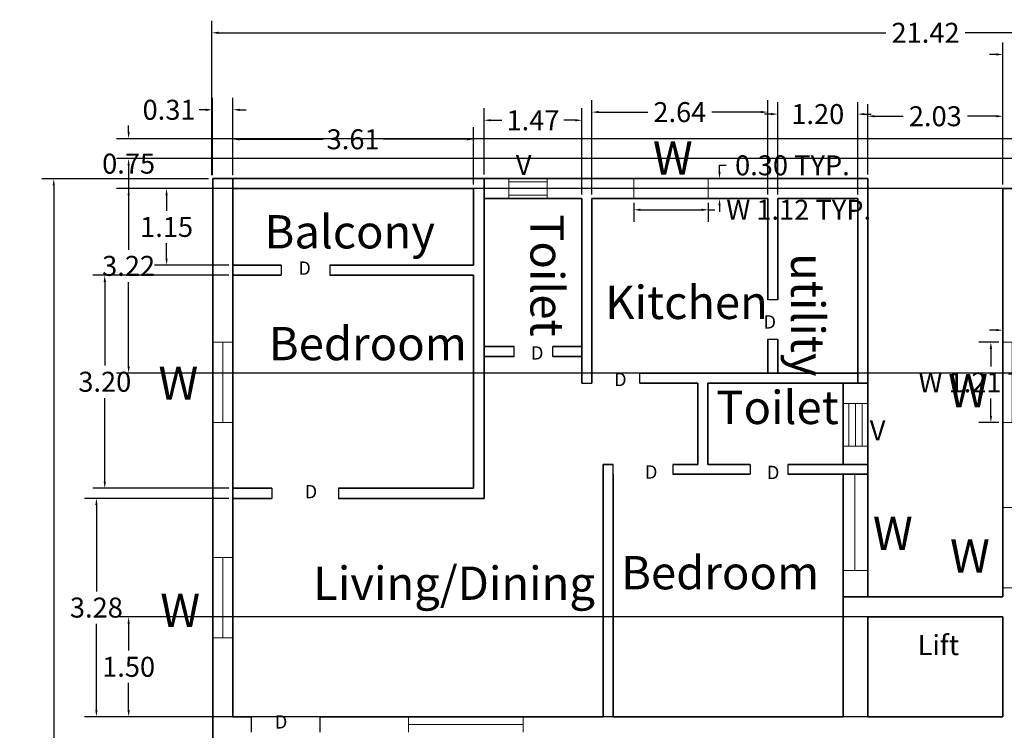
# Model space of a CAD drawing. Units: metres. Extents: x 11 to 49.6, y -23.3 to -0.8.
# Tile 3 of 5: x 11 to 25.8, y -11.5 to -0.8. Entities that reach past the tile are written whole.
import ezdxf

# ---------------------------------------------------------------- set-up
doc = ezdxf.new("R2010")
doc.units = ezdxf.units.M
doc.header["$MEASUREMENT"] = 0
for name, color, linetype, lineweight in [('A-ANNO-DIMS', 2, 'Continuous', 18), ('A-ANNO-IDEN', 3, 'Continuous', 18), ('A-AREA-IDEN', 7, 'Continuous', 18), ('A-DOOR', 3, 'Continuous', 25), ('A-FLOR-EVTR', 7, 'Continuous', 35), ('A-GLAZ', 4, 'Continuous', 18), ('A-GLAZ-VENT', 4, 'Continuous', 18), ('A-WALL', 7, 'Continuous', 35)]:
    doc.layers.add(name, color=color, linetype=linetype, lineweight=lineweight)
doc.styles.get("Standard").update_dxf_attribs({"font": 'arial.ttf'})
doc.dimstyles.get("Standard").update_dxf_attribs({"dimtxt": 0.3, "dimasz": 0.1, "dimexe": 0.18, "dimexo": 0.0625, "dimgap": 0.09, "dimtad": 0, "dimtih": 1, "dimtoh": 1, "dimzin": 0, "dimdsep": 46, "dimtxsty": 'Standard', "dimcen": 0.09, "dimadec": 0, "dimazin": 0, "dimtfac": 1, "dimtofl": 0, "dimtmove": 0, "dimatfit": 3, "dimfxl": 1, "dimtolj": 1, "dimtzin": 0, "dimarcsym": 0})

# ---------------------------------------------------------------- blocks, each defined once
blk = doc.blocks.new('*D1')
at = {"layer": 'A-ANNO-DIMS', "color": 0, "lineweight": -2, "transparency": 16777216}
for p, q in [((13.884, -3.135), (13.884, -0.816)), ((35.309, -2.864), (35.309, -0.816)), ((13.984, -0.996), (23.999, -0.996)), ((35.209, -0.996), (25.194, -0.996))]:
    blk.add_line(p, q, dxfattribs=at)
at = {"layer": 'A-ANNO-DIMS', "color": 0, "transparency": 16777216}
for points in [[(13.984, -0.979), (13.984, -1.013), (13.884, -0.996)], [(35.209, -0.979), (35.209, -1.013), (35.309, -0.996)]]:
    blk.add_solid(points, dxfattribs=at)
at = {"layer": 'Defpoints', "color": 0, "transparency": 16777216}
for p in [(35.309, -0.996), (35.309, -2.926), (13.884, -3.197)]:
    blk.add_point(p, dxfattribs=at)
at = {"layer": 'A-ANNO-DIMS', "color": 0, "transparency": 16777216, "insert": (24.597, -0.996), "char_height": 0.3, "attachment_point": 5}
blk.add_mtext('\\A1;21.42', dxfattribs=at)
blk = doc.blocks.new('*D2')
at = {"layer": 'A-ANNO-DIMS', "color": 0, "lineweight": -2, "transparency": 16777216}
for p, q in [((13.833, -3.189), (11.33, -3.189)), ((11.51, -3.289), (11.51, -12.277)), ((11.51, -21.752), (11.51, -12.764)), ((13.833, -21.852), (11.33, -21.852))]:
    blk.add_line(p, q, dxfattribs=at)
at = {"layer": 'A-ANNO-DIMS', "color": 0, "transparency": 16777216}
for points in [[(11.493, -3.289), (11.527, -3.289), (11.51, -3.189)], [(11.493, -21.752), (11.527, -21.752), (11.51, -21.852)]]:
    blk.add_solid(points, dxfattribs=at)
at = {"layer": 'Defpoints', "color": 0, "transparency": 16777216}
for p in [(13.896, -3.189), (11.51, -21.852), (13.895, -21.852)]:
    blk.add_point(p, dxfattribs=at)
at = {"layer": 'A-ANNO-DIMS', "color": 0, "transparency": 16777216, "insert": (11.51, -12.521), "char_height": 0.3, "attachment_point": 5}
blk.add_mtext('\\A1;18.66', dxfattribs=at)
blk = doc.blocks.new('*D3')
at = {"layer": 'A-ANNO-DIMS', "color": 0, "lineweight": -2, "transparency": 16777216}
for p, q in [((13.892, -3.133), (13.892, -1.972)), ((14.2, -3.133), (14.2, -1.972)), ((13.792, -2.152), (13.692, -2.152)), ((14.3, -2.152), (14.4, -2.152))]:
    blk.add_line(p, q, dxfattribs=at)
at = {"layer": 'A-ANNO-DIMS', "color": 0, "transparency": 16777216}
for points in [[(13.792, -2.136), (13.792, -2.169), (13.892, -2.152)], [(14.3, -2.136), (14.3, -2.169), (14.2, -2.152)]]:
    blk.add_solid(points, dxfattribs=at)
at = {"layer": 'Defpoints', "color": 0, "transparency": 16777216}
for p in [(13.892, -2.152), (13.892, -3.195), (14.2, -3.195)]:
    blk.add_point(p, dxfattribs=at)
at = {"layer": 'A-ANNO-DIMS', "color": 0, "transparency": 16777216, "insert": (13.241, -2.152), "char_height": 0.3, "attachment_point": 5}
blk.add_mtext('\\A1;0.31', dxfattribs=at)
blk = doc.blocks.new('*D4')
at = {"layer": 'A-ANNO-DIMS', "color": 0, "lineweight": -2, "transparency": 16777216}
for p, q in [((14.199, -3.124), (14.199, -2.415)), ((17.809, -3.274), (17.809, -2.415)), ((14.299, -2.595), (15.554, -2.595)), ((17.709, -2.595), (16.455, -2.595))]:
    blk.add_line(p, q, dxfattribs=at)
at = {"layer": 'A-ANNO-DIMS', "color": 0, "transparency": 16777216}
for points in [[(14.299, -2.579), (14.299, -2.612), (14.199, -2.595)], [(17.709, -2.579), (17.709, -2.612), (17.809, -2.595)]]:
    blk.add_solid(points, dxfattribs=at)
at = {"layer": 'Defpoints', "color": 0, "transparency": 16777216}
for p in [(17.809, -2.595), (14.199, -3.186), (17.809, -3.336)]:
    blk.add_point(p, dxfattribs=at)
at = {"layer": 'A-ANNO-DIMS', "color": 0, "transparency": 16777216, "insert": (16.004, -2.595), "char_height": 0.3, "attachment_point": 5}
blk.add_mtext('\\A1;3.61', dxfattribs=at)
blk = doc.blocks.new('*D5')
at = {"layer": 'A-ANNO-DIMS', "color": 0, "lineweight": -2, "transparency": 16777216}
for p, q in [((17.969, -3.124), (17.969, -2.13)), ((19.439, -3.424), (19.439, -2.13)), ((18.069, -2.31), (18.238, -2.31)), ((19.339, -2.31), (19.169, -2.31))]:
    blk.add_line(p, q, dxfattribs=at)
at = {"layer": 'A-ANNO-DIMS', "color": 0, "transparency": 16777216}
for points in [[(18.069, -2.293), (18.069, -2.326), (17.969, -2.31)], [(19.339, -2.293), (19.339, -2.326), (19.439, -2.31)]]:
    blk.add_solid(points, dxfattribs=at)
at = {"layer": 'Defpoints', "color": 0, "transparency": 16777216}
for p in [(19.439, -2.31), (17.969, -3.186), (19.439, -3.486)]:
    blk.add_point(p, dxfattribs=at)
at = {"layer": 'A-ANNO-DIMS', "color": 0, "transparency": 16777216, "insert": (18.704, -2.31), "char_height": 0.3, "attachment_point": 5}
blk.add_mtext('\\A1;1.47', dxfattribs=at)
blk = doc.blocks.new('*D6')
at = {"layer": 'A-ANNO-DIMS', "color": 0, "lineweight": -2, "transparency": 16777216}
for p, q in [((19.589, -3.424), (19.589, -2.007)), ((22.229, -3.424), (22.229, -2.007)), ((19.689, -2.187), (20.427, -2.187)), ((22.129, -2.187), (21.39, -2.187))]:
    blk.add_line(p, q, dxfattribs=at)
at = {"layer": 'A-ANNO-DIMS', "color": 0, "transparency": 16777216}
for points in [[(19.689, -2.17), (19.689, -2.203), (19.589, -2.187)], [(22.129, -2.17), (22.129, -2.203), (22.229, -2.187)]]:
    blk.add_solid(points, dxfattribs=at)
at = {"layer": 'Defpoints', "color": 0, "transparency": 16777216}
for p in [(22.229, -2.187), (19.589, -3.486), (22.229, -3.486)]:
    blk.add_point(p, dxfattribs=at)
at = {"layer": 'A-ANNO-DIMS', "color": 0, "transparency": 16777216, "insert": (20.909, -2.187), "char_height": 0.3, "attachment_point": 5}
blk.add_mtext('\\A1;2.64', dxfattribs=at)
blk = doc.blocks.new('*D7')
at = {"layer": 'A-ANNO-DIMS', "color": 0, "lineweight": -2, "transparency": 16777216}
for p, q in [((22.379, -3.424), (22.379, -2.037)), ((23.579, -3.424), (23.579, -2.037)), ((22.279, -2.217), (22.179, -2.217)), ((23.679, -2.217), (23.779, -2.217))]:
    blk.add_line(p, q, dxfattribs=at)
at = {"layer": 'A-ANNO-DIMS', "color": 0, "transparency": 16777216}
for points in [[(22.279, -2.2), (22.279, -2.234), (22.379, -2.217)], [(23.679, -2.2), (23.679, -2.234), (23.579, -2.217)]]:
    blk.add_solid(points, dxfattribs=at)
at = {"layer": 'Defpoints', "color": 0, "transparency": 16777216}
for p in [(23.579, -2.217), (22.379, -3.486), (23.579, -3.486)]:
    blk.add_point(p, dxfattribs=at)
at = {"layer": 'A-ANNO-DIMS', "color": 0, "transparency": 16777216, "insert": (22.979, -2.217), "char_height": 0.3, "attachment_point": 5}
blk.add_mtext('\\A1;1.20', dxfattribs=at)
blk = doc.blocks.new('*D8')
at = {"layer": 'A-ANNO-DIMS', "color": 0, "lineweight": -2, "transparency": 16777216}
for p, q in [((14.137, -3.336), (13.024, -3.336)), ((13.204, -3.436), (13.204, -3.668)), ((13.204, -4.386), (13.204, -4.154)), ((14.137, -4.486), (13.024, -4.486))]:
    blk.add_line(p, q, dxfattribs=at)
at = {"layer": 'A-ANNO-DIMS', "color": 0, "transparency": 16777216}
for points in [[(13.187, -3.436), (13.22, -3.436), (13.204, -3.336)], [(13.187, -4.386), (13.22, -4.386), (13.204, -4.486)]]:
    blk.add_solid(points, dxfattribs=at)
at = {"layer": 'Defpoints', "color": 0, "transparency": 16777216}
for p in [(14.199, -3.336), (13.204, -4.486), (14.199, -4.486)]:
    blk.add_point(p, dxfattribs=at)
at = {"layer": 'A-ANNO-DIMS', "color": 0, "transparency": 16777216, "insert": (13.204, -3.911), "char_height": 0.3, "attachment_point": 5}
blk.add_mtext('\\A1;1.15', dxfattribs=at)
blk = doc.blocks.new('*D9')
at = {"layer": 'A-ANNO-DIMS', "color": 0, "lineweight": -2, "transparency": 16777216}
for p, q in [((14.137, -4.636), (12.096, -4.636)), ((12.276, -4.736), (12.276, -5.993)), ((12.276, -7.736), (12.276, -6.48)), ((14.137, -7.836), (12.096, -7.836))]:
    blk.add_line(p, q, dxfattribs=at)
at = {"layer": 'A-ANNO-DIMS', "color": 0, "transparency": 16777216}
for points in [[(12.259, -4.736), (12.293, -4.736), (12.276, -4.636)], [(12.259, -7.736), (12.293, -7.736), (12.276, -7.836)]]:
    blk.add_solid(points, dxfattribs=at)
at = {"layer": 'Defpoints', "color": 0, "transparency": 16777216}
for p in [(14.199, -4.636), (12.276, -7.836), (14.199, -7.836)]:
    blk.add_point(p, dxfattribs=at)
at = {"layer": 'A-ANNO-DIMS', "color": 0, "transparency": 16777216, "insert": (12.276, -6.236), "char_height": 0.3, "attachment_point": 5}
blk.add_mtext('\\A1;3.20', dxfattribs=at)
blk = doc.blocks.new('*D10')
at = {"layer": 'A-ANNO-DIMS', "color": 0, "lineweight": -2, "transparency": 16777216}
for p, q in [((14.137, -7.987), (11.97, -7.987)), ((12.15, -8.087), (12.15, -9.383)), ((12.15, -11.166), (12.15, -9.87)), ((14.137, -11.266), (11.97, -11.266))]:
    blk.add_line(p, q, dxfattribs=at)
at = {"layer": 'A-ANNO-DIMS', "color": 0, "transparency": 16777216}
for points in [[(12.134, -8.087), (12.167, -8.087), (12.15, -7.987)], [(12.134, -11.166), (12.167, -11.166), (12.15, -11.266)]]:
    blk.add_solid(points, dxfattribs=at)
at = {"layer": 'Defpoints', "color": 0, "transparency": 16777216}
for p in [(14.199, -7.987), (12.15, -11.266), (14.199, -11.266)]:
    blk.add_point(p, dxfattribs=at)
at = {"layer": 'A-ANNO-DIMS', "color": 0, "transparency": 16777216, "insert": (12.15, -9.627), "char_height": 0.3, "attachment_point": 5}
blk.add_mtext('\\A1;3.28', dxfattribs=at)
blk = doc.blocks.new('*D12')
at = {"layer": 'A-ANNO-DIMS', "color": 0, "lineweight": -2, "transparency": 16777216}
for p, q in [((23.729, -3.124), (23.729, -2.069)), ((25.759, -3.274), (25.759, -2.069)), ((23.829, -2.249), (24.262, -2.249)), ((25.659, -2.249), (25.226, -2.249))]:
    blk.add_line(p, q, dxfattribs=at)
at = {"layer": 'A-ANNO-DIMS', "color": 0, "transparency": 16777216}
for points in [[(23.829, -2.232), (23.829, -2.266), (23.729, -2.249)], [(25.659, -2.232), (25.659, -2.266), (25.759, -2.249)]]:
    blk.add_solid(points, dxfattribs=at)
at = {"layer": 'Defpoints', "color": 0, "transparency": 16777216}
for p in [(25.759, -2.249), (23.729, -3.186), (25.759, -3.336)]:
    blk.add_point(p, dxfattribs=at)
at = {"layer": 'A-ANNO-DIMS', "color": 0, "transparency": 16777216, "insert": (24.744, -2.249), "char_height": 0.3, "attachment_point": 5}
blk.add_mtext('\\A1;2.03', dxfattribs=at)
blk = doc.blocks.new('WIN-1119-D300')
for p, q in [((0, 0.3), (0, 0)), ((1.119, 0.3), (1.119, 0)), ((0, 0.15), (1.119, 0.15))]:
    blk.add_line(p, q)
blk = doc.blocks.new('WIN-1207-D300')
for p, q in [((0.3, 1.207), (0, 1.207)), ((0.15, 1.207), (0.15, 0)), ((0, 0), (0.3, 0))]:
    blk.add_line(p, q)
blk = doc.blocks.new('WIN-1207-D290')
for p, q in [((0.29, 1.207), (0, 1.207)), ((0.14, 1.207), (0.14, 0)), ((0, 0), (0.29, 0))]:
    blk.add_line(p, q)
blk = doc.blocks.new('WIN-1724-D230')
for p, q in [((0, 0.23), (0, 0)), ((1.724, 0.23), (1.724, 0)), ((0, 0.115), (1.724, 0.115))]:
    blk.add_line(p, q)
blk = doc.blocks.new('VENT-572')
for p, q in [((0, 0.3), (0, 0)), ((0.572, 0.3), (0.572, 0)), ((0, 0.25), (0.572, 0.25)), ((0, 0.15), (0.572, 0.15)), ((0, 0.05), (0.572, 0.05))]:
    blk.add_line(p, q)
blk = doc.blocks.new('*D34')
at = {"layer": 'A-ANNO-DIMS', "color": 0, "lineweight": -2, "transparency": 16777216}
for p, q in [((20.217, -3.549), (20.217, -3.834)), ((20.317, -3.654), (21.236, -3.654)), ((21.336, -3.549), (21.336, -3.834)), ((21.336, -3.654), (21.436, -3.654))]:
    blk.add_line(p, q, dxfattribs=at)
at = {"layer": 'A-ANNO-DIMS', "color": 0, "transparency": 16777216}
for points in [[(20.317, -3.637), (20.317, -3.671), (20.217, -3.654)], [(21.236, -3.637), (21.236, -3.671), (21.336, -3.654)]]:
    blk.add_solid(points, dxfattribs=at)
at = {"layer": 'Defpoints', "color": 0, "transparency": 16777216}
for p in [(20.217, -3.486), (21.336, -3.486), (21.336, -3.654)]:
    blk.add_point(p, dxfattribs=at)
at = {"layer": 'A-ANNO-DIMS', "color": 0, "transparency": 16777216, "insert": (22.693, -3.654), "char_height": 0.3, "attachment_point": 5}
blk.add_mtext('\\A1;W 1.12 TYP.', dxfattribs=at)
blk = doc.blocks.new('*D35')
at = {"layer": 'A-ANNO-DIMS', "color": 0, "lineweight": -2, "transparency": 16777216}
for p, q in [((21.504, -3.086), (21.504, -2.986)), ((21.504, -2.986), (21.604, -2.986)), ((21.399, -3.186), (21.684, -3.186)), ((21.399, -3.486), (21.684, -3.486)), ((21.504, -3.586), (21.504, -3.686))]:
    blk.add_line(p, q, dxfattribs=at)
at = {"layer": 'A-ANNO-DIMS', "color": 0, "transparency": 16777216}
for points in [[(21.487, -3.086), (21.521, -3.086), (21.504, -3.186)], [(21.487, -3.586), (21.521, -3.586), (21.504, -3.486)]]:
    blk.add_solid(points, dxfattribs=at)
at = {"layer": 'Defpoints', "color": 0, "transparency": 16777216}
for p in [(21.336, -3.186), (21.504, -3.186), (21.336, -3.486)]:
    blk.add_point(p, dxfattribs=at)
at = {"layer": 'A-ANNO-DIMS', "color": 0, "transparency": 16777216, "insert": (22.599, -2.986), "char_height": 0.3, "attachment_point": 5}
blk.add_mtext('\\A1;0.30 TYP.', dxfattribs=at)
blk = doc.blocks.new('*D36')
at = {"layer": 'A-ANNO-DIMS', "color": 0, "lineweight": -2, "transparency": 16777216}
for p, q in [((25.697, -5.642), (25.398, -5.642)), ((25.578, -5.742), (25.578, -6.005)), ((25.578, -6.749), (25.578, -6.486)), ((25.697, -6.849), (25.398, -6.849))]:
    blk.add_line(p, q, dxfattribs=at)
at = {"layer": 'A-ANNO-DIMS', "color": 0, "transparency": 16777216}
for points in [[(25.561, -5.742), (25.595, -5.742), (25.578, -5.642)], [(25.561, -6.749), (25.595, -6.749), (25.578, -6.849)]]:
    blk.add_solid(points, dxfattribs=at)
at = {"layer": 'Defpoints', "color": 0, "transparency": 16777216}
for p in [(25.578, -5.642), (25.759, -5.642), (25.759, -6.849)]:
    blk.add_point(p, dxfattribs=at)
at = {"layer": 'A-ANNO-DIMS', "color": 0, "transparency": 16777216, "insert": (25.578, -6.246), "char_height": 0.3, "attachment_point": 5}
blk.add_mtext('\\A1;W 1.21 TYP.', dxfattribs=at)
blk = doc.blocks.new('*D37')
at = {"layer": 'A-ANNO-DIMS', "color": 0, "lineweight": -2, "transparency": 16777216}
for p, q in [((25.759, -5.579), (25.759, -5.281)), ((26.05, -5.579), (26.05, -5.281)), ((25.659, -5.461), (25.559, -5.461)), ((26.15, -5.461), (26.25, -5.461))]:
    blk.add_line(p, q, dxfattribs=at)
at = {"layer": 'A-ANNO-DIMS', "color": 0, "transparency": 16777216}
for points in [[(25.659, -5.444), (25.659, -5.477), (25.759, -5.461)], [(26.15, -5.444), (26.15, -5.477), (26.05, -5.461)]]:
    blk.add_solid(points, dxfattribs=at)
at = {"layer": 'Defpoints', "color": 0, "transparency": 16777216}
for p in [(26.05, -5.461), (25.759, -5.642), (26.05, -5.642)]:
    blk.add_point(p, dxfattribs=at)
at = {"layer": 'A-ANNO-DIMS', "color": 0, "transparency": 16777216, "insert": (27.244, -5.461), "char_height": 0.3, "attachment_point": 5}
blk.add_mtext('\\A1;0.29 TYP.', dxfattribs=at)
blk = doc.blocks.new('*D57')
at = {"layer": 'A-ANNO-DIMS', "color": 0, "lineweight": -2, "transparency": 16777216}
for p, q in [((33.747, -2.886), (12.454, -2.886)), ((12.634, -2.986), (12.634, -4.253)), ((12.634, -6.006), (12.634, -4.739)), ((33.747, -6.106), (12.454, -6.106))]:
    blk.add_line(p, q, dxfattribs=at)
at = {"layer": 'A-ANNO-DIMS', "color": 0, "transparency": 16777216}
for points in [[(12.618, -2.986), (12.651, -2.986), (12.634, -2.886)], [(12.618, -6.006), (12.651, -6.006), (12.634, -6.106)]]:
    blk.add_solid(points, dxfattribs=at)
at = {"layer": 'Defpoints', "color": 0, "transparency": 16777216}
for p in [(33.809, -2.886), (12.634, -6.106), (33.809, -6.106)]:
    blk.add_point(p, dxfattribs=at)
at = {"layer": 'A-ANNO-DIMS', "color": 0, "transparency": 16777216, "insert": (12.634, -4.496), "char_height": 0.3, "attachment_point": 5}
blk.add_mtext('\\A1;3.22', dxfattribs=at)
blk = doc.blocks.new('*D60')
at = {"layer": 'A-ANNO-DIMS', "color": 0, "lineweight": -2, "transparency": 16777216}
for p, q in [((25.697, -9.766), (12.454, -9.766)), ((12.634, -9.866), (12.634, -10.273)), ((12.634, -11.166), (12.634, -10.759)), ((25.697, -11.266), (12.454, -11.266))]:
    blk.add_line(p, q, dxfattribs=at)
at = {"layer": 'A-ANNO-DIMS', "color": 0, "transparency": 16777216}
for points in [[(12.618, -9.866), (12.651, -9.866), (12.634, -9.766)], [(12.618, -11.166), (12.651, -11.166), (12.634, -11.266)]]:
    blk.add_solid(points, dxfattribs=at)
at = {"layer": 'Defpoints', "color": 0, "transparency": 16777216}
for p in [(25.759, -9.766), (12.634, -11.266), (25.759, -11.266)]:
    blk.add_point(p, dxfattribs=at)
at = {"layer": 'A-ANNO-DIMS', "color": 0, "transparency": 16777216, "insert": (12.634, -10.516), "char_height": 0.3, "attachment_point": 5}
blk.add_mtext('\\A1;1.50', dxfattribs=at)
blk = doc.blocks.new('*D61')
at = {"layer": 'A-ANNO-DIMS', "color": 0, "lineweight": -2, "transparency": 16777216}
for p, q in [((25.759, -3.274), (25.759, -1.141)), ((26.9, -2.524), (26.9, -1.141)), ((25.659, -1.321), (25.559, -1.321)), ((27, -1.321), (27.1, -1.321))]:
    blk.add_line(p, q, dxfattribs=at)
at = {"layer": 'A-ANNO-DIMS', "color": 0, "transparency": 16777216}
for points in [[(25.659, -1.304), (25.659, -1.338), (25.759, -1.321)], [(27, -1.304), (27, -1.338), (26.9, -1.321)]]:
    blk.add_solid(points, dxfattribs=at)
at = {"layer": 'Defpoints', "color": 0, "transparency": 16777216}
for p in [(25.759, -1.321), (26.9, -2.586), (25.759, -3.336)]:
    blk.add_point(p, dxfattribs=at)
at = {"layer": 'A-ANNO-DIMS', "color": 0, "transparency": 16777216, "insert": (26.329, -1.321), "char_height": 0.3, "attachment_point": 5}
blk.add_mtext('\\A1;1.14', dxfattribs=at)
blk = doc.blocks.new('*D62')
at = {"layer": 'A-ANNO-DIMS', "color": 0, "lineweight": -2, "transparency": 16777216}
for p, q in [((12.634, -2.486), (12.634, -2.386)), ((26.837, -2.586), (12.454, -2.586)), ((26.837, -3.336), (12.454, -3.336)), ((12.634, -3.436), (12.634, -3.536))]:
    blk.add_line(p, q, dxfattribs=at)
at = {"layer": 'A-ANNO-DIMS', "color": 0, "transparency": 16777216}
for points in [[(12.618, -2.486), (12.651, -2.486), (12.634, -2.586)], [(12.618, -3.436), (12.651, -3.436), (12.634, -3.336)]]:
    blk.add_solid(points, dxfattribs=at)
at = {"layer": 'Defpoints', "color": 0, "transparency": 16777216}
for p in [(26.9, -2.586), (12.634, -3.336), (26.9, -3.336)]:
    blk.add_point(p, dxfattribs=at)
at = {"layer": 'A-ANNO-DIMS', "color": 0, "transparency": 16777216, "insert": (12.634, -2.961), "char_height": 0.3, "attachment_point": 5}
blk.add_mtext('\\A1;0.75', dxfattribs=at)

msp = doc.modelspace()

# ---------------------------------------------------------------- linework, layer by layer
at = {"layer": 'A-DOOR'}
for p, q in [((14.924, -4.486), (14.924, -4.636)), ((15.657, -4.486), (15.657, -4.636)), ((22.379, -5.005), (22.229, -5.005)), ((22.229, -5.596), (22.379, -5.596)), ((18.42, -5.856), (18.42, -5.706)), ((19, -5.856), (19, -5.706)), ((20.309, -6.256), (20.309, -6.106)), ((19.439, -6.256), (19.589, -6.256)), ((19.909, -7.626), (19.909, -7.476)), ((20.803, -7.476), (20.803, -7.626)), ((21.964, -7.476), (21.964, -7.626)), ((22.529, -7.476), (22.529, -7.626)), ((14.785, -7.836), (14.785, -7.987)), ((15.787, -7.836), (15.787, -7.987)), ((14.474, -11.266), (14.474, -11.496)), ((15.505, -11.266), (15.505, -11.496))]:
    msp.add_line(p, q, dxfattribs=at)
at = {"layer": 'A-FLOR-EVTR'}
for p, q in [((23.359, -9.466), (25.759, -9.466)), ((23.729, -9.766), (25.759, -9.766)), ((23.729, -9.766), (23.729, -11.266)), ((25.759, -9.766), (25.759, -11.266)), ((23.729, -11.266), (25.759, -11.266)), ((23.729, -11.266), (23.829, -11.266))]:
    msp.add_line(p, q, dxfattribs=at)
at = {"layer": 'A-GLAZ'}
for p, q in [((23.535, -7.626), (23.535, -9.069)), ((23.729, -9.069), (23.359, -9.069))]:
    msp.add_line(p, q, dxfattribs=at)
at = {"layer": 'A-GLAZ-VENT'}
for p, q in [((23.359, -6.561), (23.729, -6.561)), ((23.444, -6.561), (23.444, -7.202)), ((23.444, -6.561), (23.444, -7.202)), ((23.444, -6.561), (23.444, -7.202)), ((23.544, -6.561), (23.544, -7.202)), ((23.644, -6.561), (23.644, -7.202)), ((23.359, -7.202), (23.729, -7.202))]:
    msp.add_line(p, q, dxfattribs=at)
at = {"layer": 'A-WALL'}
for p, q in [((13.899, -3.186), (13.899, -14.166)), ((13.899, -3.186), (23.729, -3.186)), ((14.199, -3.186), (14.199, -11.266)), ((17.969, -3.186), (17.969, -5.706)), ((23.729, -3.186), (23.729, -7.476)), ((14.199, -3.336), (14.199, -4.486)), ((14.199, -3.336), (17.809, -3.336)), ((17.809, -3.336), (17.809, -4.486)), ((25.759, -3.336), (25.759, -9.466)), ((25.759, -3.336), (26.9, -3.336)), ((17.969, -3.486), (19.439, -3.486)), ((19.439, -3.486), (19.439, -5.706)), ((19.589, -3.486), (19.589, -6.106)), ((19.589, -3.486), (22.229, -3.486)), ((22.229, -3.486), (22.229, -5.005)), ((22.379, -3.486), (22.379, -5.005)), ((22.379, -3.486), (23.579, -3.486)), ((23.579, -3.486), (23.579, -6.256)), ((14.199, -4.486), (14.924, -4.486)), ((15.657, -4.486), (17.809, -4.486)), ((14.199, -4.636), (14.924, -4.636)), ((14.199, -4.636), (14.199, -11.266)), ((15.657, -4.636), (17.809, -4.636)), ((17.809, -4.636), (17.809, -7.836)), ((22.229, -5.596), (22.229, -6.106)), ((22.379, -5.596), (22.379, -6.106)), ((17.969, -5.656), (17.969, -7.987)), ((17.969, -5.706), (18.42, -5.706)), ((19, -5.706), (19.439, -5.706)), ((19.439, -5.656), (19.439, -6.256)), ((19.589, -5.656), (19.589, -6.256)), ((17.969, -5.856), (18.42, -5.856)), ((19, -5.856), (19.439, -5.856)), ((20.309, -6.106), (22.229, -6.106)), ((22.229, -6.106), (23.579, -6.106)), ((20.309, -6.256), (21.179, -6.256)), ((21.179, -6.256), (21.179, -7.476)), ((21.329, -6.256), (23.729, -6.256)), ((21.329, -6.256), (21.329, -7.476)), ((23.359, -6.256), (23.359, -7.476)), ((19.759, -7.476), (19.909, -7.476)), ((19.759, -7.476), (19.759, -11.266)), ((20.803, -7.476), (21.179, -7.476)), ((21.329, -7.476), (21.964, -7.476)), ((22.529, -7.476), (23.729, -7.476)), ((23.729, -7.476), (23.729, -9.466)), ((19.759, -7.626), (19.759, -11.266)), ((19.909, -7.626), (19.909, -11.266)), ((20.803, -7.626), (21.964, -7.626)), ((22.529, -7.626), (23.729, -7.626)), ((23.359, -7.626), (23.359, -11.266)), ((14.199, -7.836), (14.785, -7.836)), ((15.787, -7.836), (17.809, -7.836)), ((14.199, -7.987), (14.785, -7.987)), ((15.787, -7.987), (17.969, -7.987)), ((14.199, -11.266), (14.474, -11.266)), ((15.505, -11.266), (19.759, -11.266)), ((15.505, -11.266), (19.759, -11.266)), ((19.909, -11.266), (20.719, -11.266)), ((20.009, -11.266), (23.359, -11.266)), ((20.719, -11.266), (23.359, -11.266))]:
    msp.add_line(p, q, dxfattribs=at)

# ---------------------------------------------------------------- block references
at = {"layer": 'A-GLAZ'}
for name, p in [('WIN-1119-D300', (20.217, -3.486)), ('WIN-1207-D300', (13.899, -6.849)), ('WIN-1207-D290', (25.759, -6.849)), ('WIN-1724-D230', (16.834, -11.496))]:
    msp.add_blockref(name, p, dxfattribs=at)
at = {"layer": 'A-GLAZ', "rotation": 180}
for name, p in [('WIN-1207-D290', (26.05, -8.123)), ('WIN-1207-D300', (14.199, -8.873))]:
    msp.add_blockref(name, p, dxfattribs=at)
at = {"layer": 'A-GLAZ-VENT'}
msp.add_blockref('VENT-572', (18.343, -3.486), dxfattribs=at)

# ---------------------------------------------------------------- texts
at = {"layer": 'A-ANNO-IDEN', "attachment_point": 1}
for s, width, insert, char_height in [('W', 1.41386, (20.504, -2.624), 0.5), ('V', 0.1, (18.446, -2.83), 0.3), ('D', 0.77129, (15.182, -4.43), 0.2), ('D', 0.77129, (22.165, -5.237), 0.2), ('D', 0.77129, (18.674, -5.703), 0.2), ('W', 1.41386, (13.081, -6.007), 0.5), ('D', 0.77129, (19.922, -6.102), 0.2), ('W', 1.41386, (24.936, -6.12), 0.5), ('V', 0.1, (23.76, -6.817), 0.3), ('D', 0.77129, (20.385, -7.491), 0.2), ('D', 0.77129, (22.216, -7.498), 0.2), ('D', 0.77129, (15.277, -7.786), 0.2), ('W', 1.41386, (23.807, -8.262), 0.5), ('W', 1.41386, (24.964, -8.601), 0.5), ('W', 1.41386, (13.109, -9.418), 0.5), ('D', 0.77129, (14.829, -11.243), 0.2)]:
    msp.add_mtext_dynamic_manual_height_columns(s, width=width, gutter_width=0.5, heights=[0], dxfattribs=dict(at, insert=insert, char_height=char_height))
at = {"layer": 'A-AREA-IDEN', "attachment_point": 1}
for s, width, gutter_width, heights, insert, char_height in [('Balcony', 2.63335, 1, [0], (14.674, -3.734), 0.5), ('Kitchen', 2.63335, 1, [0], (19.788, -4.794), 0.5), ('Bedroom', 2.63335, 1, [0], (14.739, -5.413), 0.5), ('Toilet', 2.63335, 1, [0], (21.456, -6.371), 0.5), ('Bedroom', 2.63335, 1, [0], (20.027, -8.853), 0.5), ('Living/Dining', 2.63335, 1, [0], (15.404, -9.011), 0.5), ('Lift', 1.16012, 0.5, [0.103], (24.478, -10.04), 0.3)]:
    msp.add_mtext_dynamic_manual_height_columns(s, width=width, gutter_width=gutter_width, heights=heights, dxfattribs=dict(at, insert=insert, char_height=char_height))
at = {"layer": 'A-AREA-IDEN', "char_height": 0.5, "attachment_point": 1, "rotation": 270}
for s, insert in [('Toilet', (19.166, -3.72)), ('utility', (23.079, -4.306))]:
    msp.add_mtext_dynamic_manual_height_columns(s, width=2.63335, gutter_width=1, heights=[0], dxfattribs=dict(at, insert=insert))

# ---------------------------------------------------------------- dimensions: what is measured, and where the dimension line sits
at = {"layer": 'A-ANNO-DIMS'}
for base, p1, p2, override, picture, middle in [((35.3087, -0.9961), (13.8844, -3.197), (35.3087, -2.9263), {"dimclrd": 0, "dimclre": 0, "dimclrt": 0}, '*D1', (24.5966, -0.9961)), ((25.759, -1.321), (26.9, -2.586), (25.759, -3.336), {"dimdec": 2, "dimlfac": 1, "dimrnd": 0, "dimzin": 0, "dimdsep": 46, "dimlunit": 2}, '*D61', (26.329, -1.321)), ((13.892, -2.152), (14.2, -3.195), (13.892, -3.195), {"dimclrd": 0, "dimclre": 0, "dimclrt": 0}, '*D3', (13.241, -2.152)), ((22.229, -2.187), (19.589, -3.486), (22.229, -3.486), {"dimclrd": 0, "dimclre": 0, "dimclrt": 0}, '*D6', (20.909, -2.187)), ((23.579, -2.217), (22.379, -3.486), (23.579, -3.486), {"dimclrd": 0, "dimclre": 0, "dimclrt": 0}, '*D7', (22.979, -2.217)), ((25.759, -2.249), (23.729, -3.186), (25.759, -3.336), {"dimclrd": 0, "dimclre": 0, "dimclrt": 0}, '*D12', (24.744, -2.249)), ((19.439, -2.31), (17.969, -3.186), (19.439, -3.486), {"dimclrd": 0, "dimclre": 0, "dimclrt": 0}, '*D5', (18.704, -2.31)), ((17.809, -2.595), (14.199, -3.186), (17.809, -3.336), {"dimclrd": 0, "dimclre": 0, "dimclrt": 0}, '*D4', (16.004, -2.595))]:
    dim = msp.add_linear_dim(base=base, p1=p1, p2=p2, dimstyle='Standard', override=override, dxfattribs=at)
    dim.commit()
    dim.dimension.update_dxf_attribs({"geometry": picture, "text_midpoint": middle})
for base, p1, p2, override, picture, middle in [((12.634, -3.336), (26.9, -2.586), (26.9, -3.336), {"dimdec": 2, "dimlfac": 1, "dimrnd": 0, "dimzin": 0, "dimdsep": 46, "dimlunit": 2}, '*D62', (12.634, -2.961)), ((12.634, -6.106), (33.809, -2.886), (33.809, -6.106), {"dimdec": 2, "dimlfac": 1, "dimrnd": 0, "dimzin": 0, "dimdsep": 46, "dimlunit": 2}, '*D57', (12.634, -4.496)), ((11.51, -21.852), (13.896, -3.189), (13.895, -21.852), {"dimclrd": 0, "dimclre": 0, "dimclrt": 0}, '*D2', (11.51, -12.521)), ((13.204, -4.486), (14.199, -3.336), (14.199, -4.486), {"dimclrd": 0, "dimclre": 0, "dimclrt": 0}, '*D8', (13.204, -3.911)), ((12.276, -7.836), (14.199, -4.636), (14.199, -7.836), {"dimclrd": 0, "dimclre": 0, "dimclrt": 0}, '*D9', (12.276, -6.236)), ((12.15, -11.266), (14.199, -7.987), (14.199, -11.266), {"dimclrd": 0, "dimclre": 0, "dimclrt": 0}, '*D10', (12.15, -9.627)), ((12.634, -11.266), (25.759, -9.766), (25.759, -11.266), {"dimdec": 2, "dimlfac": 1, "dimrnd": 0, "dimzin": 0, "dimdsep": 46, "dimlunit": 2}, '*D60', (12.634, -10.516))]:
    dim = msp.add_linear_dim(base=base, p1=p1, p2=p2, angle=90, dimstyle='Standard', override=override, dxfattribs=at)
    dim.commit()
    dim.dimension.update_dxf_attribs({"geometry": picture, "text_midpoint": middle})
for base, p1, p2, text, picture, middle in [((21.504, -3.186), (21.336, -3.486), (21.336, -3.186), '<> TYP.', '*D35', (22.599, -2.986)), ((25.578, -5.642), (25.759, -6.849), (25.759, -5.642), 'W <> TYP.', '*D36', (25.578, -6.246))]:
    dim = msp.add_linear_dim(base=base, p1=p1, p2=p2, angle=90, text=text, dimstyle='Standard', override={"dimdec": 2, "dimlfac": 1, "dimrnd": 0, "dimzin": 0, "dimdsep": 46, "dimlunit": 2}, dxfattribs=at)
    dim.commit()
    dim.dimension.update_dxf_attribs({"geometry": picture, "text_midpoint": middle})
for base, p1, p2, text, picture, middle in [((21.336, -3.654), (20.217, -3.486), (21.336, -3.486), 'W <> TYP.', '*D34', (22.693, -3.654)), ((26.05, -5.461), (25.759, -5.642), (26.05, -5.642), '<> TYP.', '*D37', (27.244, -5.461))]:
    dim = msp.add_linear_dim(base=base, p1=p1, p2=p2, text=text, dimstyle='Standard', override={"dimdec": 2, "dimlfac": 1, "dimrnd": 0, "dimzin": 0, "dimdsep": 46, "dimlunit": 2}, dxfattribs=at)
    dim.commit()
    dim.dimension.update_dxf_attribs({"geometry": picture, "text_midpoint": middle})

doc.saveas('drawing.dxf')
